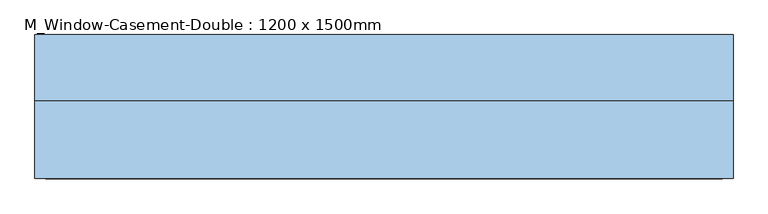
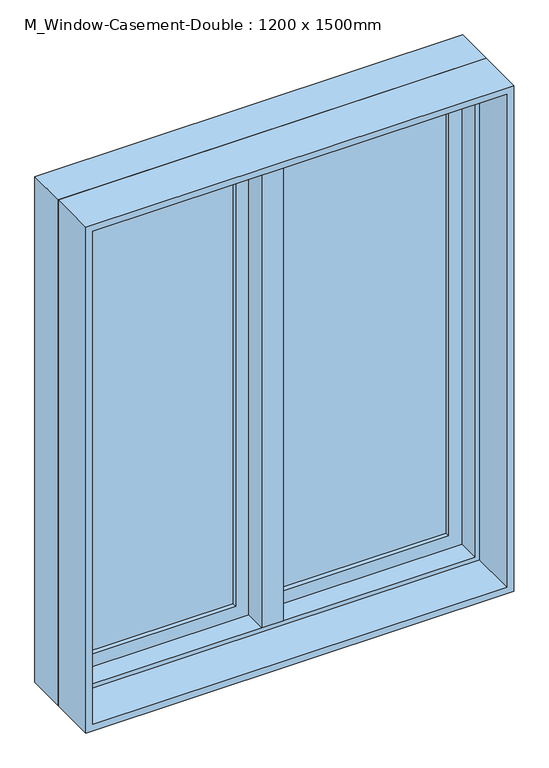
"""IFC4 building model written with IfcOpenShell, lengths in millimetres: window geometry, M_Window-Casement-Double : 1200 x 1500mm."""

from ifc_helpers import new_model, si_unit, frame, origin, place, context, project, spatial, polyline, outline, extrude, faceted_brep, source, transform, mapped, element, save


def m_window_casement_double_1200_x_1500mm_04159c99(model_context):
    return source(origin(), model_context, "Body", "SolidModel", [
        faceted_brep([(9.525, 133.35, 2387.3), (-9.525, 133.35, 2387.3), (-9.525, 82.55, 2387.3), (9.525, 82.55, 2387.3), (9.525, 133.35, 912.7), (9.525, 82.55, 912.7), (-9.525, 82.55, 912.7), (-9.525, 133.35, 912.7), (-9.525, 82.55, 931.75), (-9.525, 82.55, 2368.25), (-30.1625, 82.55, 931.75), (-30.1625, 82.55, 2368.25), (-30.1625, 19.05, 931.75), (-30.1625, 19.05, 2368.25), (30.1625, 19.05, 931.75), (30.1625, 19.05, 2368.25), (30.1625, 82.55, 931.75), (30.1625, 82.55, 2368.25), (9.525, 82.55, 931.75), (9.525, 82.55, 2368.25)], [[[0, 1, 2, 3]], [[4, 5, 6, 7]], [[1, 0, 4, 7]], [[2, 1, 7, 6, 8, 9]], [[9, 8, 10, 11]], [[11, 10, 12, 13]], [[13, 12, 14, 15]], [[15, 14, 16, 17]], [[17, 16, 18, 19]], [[0, 3, 19, 18, 5, 4]], [[18, 8, 6, 5]], [[9, 19, 3, 2]], [[8, 18, 16, 14, 12, 10]], [[19, 9, 11, 13, 15, 17]]]),
        extrude(outline(polyline([(-66.675, 114.3), (-66.675, 107.95), (-530.15, 107.95), (-530.15, 114.3), (-66.675, 114.3)])), frame((0.0, 0.0, 969.85), z_axis=(0.0, 0.0, 1.0), x_axis=(1.0, 0.0, 0.0)), (0.0, 0.0, 1.0), 1360.3),
        extrude(outline(polyline([(-530.15, 95.25), (-530.15, 101.6), (-66.675, 101.6), (-66.675, 95.25), (-530.15, 95.25)])), frame((0.0, 0.0, 969.85), z_axis=(0.0, 0.0, 1.0), x_axis=(1.0, 0.0, 0.0)), (0.0, 0.0, 1.0), 1360.3),
        extrude(outline(polyline([(530.15, 114.3), (530.15, 107.95), (66.675, 107.95), (66.675, 114.3), (530.15, 114.3)])), frame((0.0, 0.0, 969.85), z_axis=(0.0, 0.0, 1.0), x_axis=(1.0, 0.0, 0.0)), (0.0, 0.0, 1.0), 1360.3),
        extrude(outline(polyline([(66.675, 95.25), (66.675, 101.6), (530.15, 101.6), (530.15, 95.25), (66.675, 95.25)])), frame((0.0, 0.0, 969.85), z_axis=(0.0, 0.0, 1.0), x_axis=(1.0, 0.0, 0.0)), (0.0, 0.0, 1.0), 1360.3),
        extrude(outline(polyline([(2387.3, -587.3), (912.7, -587.3), (912.7, -9.525), (2387.3, -9.525), (2387.3, -587.3)]), holes=[polyline([(2330.15, -66.675), (969.85, -66.675), (969.85, -530.15), (2330.15, -530.15), (2330.15, -66.675)])]), frame((0.0, 82.55, 0.0), z_axis=(0.0, 1.0, 0.0), x_axis=(0.0, 0.0, 1.0)), (0.0, 0.0, 1.0), 44.45),
        extrude(outline(polyline([(912.7, 587.3), (2387.3, 587.3), (2387.3, 9.525), (912.7, 9.525), (912.7, 587.3)]), holes=[polyline([(969.85, 66.675), (2330.15, 66.675), (2330.15, 530.15), (969.85, 530.15), (969.85, 66.675)])]), frame((0.0, 82.55, 0.0), z_axis=(0.0, 1.0, 0.0), x_axis=(0.0, 0.0, 1.0)), (0.0, 0.0, 1.0), 44.45),
        extrude(outline(polyline([(2400.0, -600.0), (900.0, -600.0), (900.0, 600.0), (2400.0, 600.0), (2400.0, -600.0)]), holes=[polyline([(2380.95, 580.95), (919.05, 580.95), (919.05, -580.95), (2380.95, -580.95), (2380.95, 580.95)])]), frame((0.0, -114.3, 0.0), z_axis=(0.0, 1.0, 0.0), x_axis=(0.0, 0.0, 1.0)), (0.0, 0.0, 1.0), 133.35),
        faceted_brep([(568.25, 82.55, 2368.25), (568.25, 19.05, 2368.25), (-568.25, 19.05, 2368.25), (-568.25, 82.55, 2368.25), (587.3, 133.35, 2387.3), (587.3, 82.55, 2387.3), (-587.3, 82.55, 2387.3), (-587.3, 133.35, 2387.3), (600.0, 19.05, 2400.0), (600.0, 133.35, 2400.0), (-600.0, 133.35, 2400.0), (-600.0, 19.05, 2400.0), (-568.25, 19.05, 931.75), (-568.25, 82.55, 931.75), (-587.3, 82.55, 912.7), (-587.3, 133.35, 912.7), (-600.0, 133.35, 900.0), (-600.0, 19.05, 900.0), (568.25, 19.05, 931.75), (568.25, 82.55, 931.75), (587.3, 82.55, 912.7), (587.3, 133.35, 912.7), (600.0, 133.35, 900.0), (600.0, 19.05, 900.0)], [[[0, 1, 2, 3]], [[4, 5, 6, 7]], [[8, 9, 10, 11]], [[3, 2, 12, 13]], [[7, 6, 14, 15]], [[11, 10, 16, 17]], [[13, 12, 18, 19]], [[15, 14, 20, 21]], [[17, 16, 22, 23]], [[11, 17, 23, 8], [1, 18, 12, 2]], [[19, 18, 1, 0]], [[5, 20, 14, 6], [3, 13, 19, 0]], [[21, 20, 5, 4]], [[23, 22, 9, 8]], [[9, 22, 16, 10], [7, 15, 21, 4]]]),
    ])


if __name__ == "__main__":
    model = new_model("IFC4")
    model_context = context("Model", 3, world=origin())
    ifc_project = project(units=[si_unit("LENGTHUNIT", "METRE", prefix="MILLI")], contexts=[model_context])
    site = spatial("IfcSite", under=ifc_project)
    building = spatial("IfcBuilding", under=site)
    placement = place(None, origin())
    m_window_casement_double_1200_x_1500mm_shape = m_window_casement_double_1200_x_1500mm_04159c99(model_context)
    element("IfcWindow", 1, ObjectType="M_Window-Casement-Double : 1200 x 1500mm", at=placement, inside=building, context=model_context, shape_type="MappedRepresentation", body=[
        mapped(m_window_casement_double_1200_x_1500mm_shape, transform((0.0, 0.0, 0.0), x_axis=(1.0, 0.0, 0.0), y_axis=(0.0, 1.0, 0.0), z_axis=(0.0, 0.0, 1.0))),
    ])
    save(model, "model.ifc")

# Revit data of these elements
# Type "M_Window-Casement-Double : 1200 x 1500mm"
#   Type Mark = "25"
#   Fire Rating = "0.5h"
#   Assembly Code = "B2020100"
#   Analytic Construction = "Double glazing - domestic"
#   Frame Extension [instance default] = 0.020833 ft
#   Window Inset [instance default] = 0.0 ft
#   Wall Thickness [instance default] = 0.492126 ft
#   Interior Wall Closure [instance default] = 0.179626 ft
#   Half Width = 1.968504 ft
#   Visual Light Transmittance = 0.81
#   Thermal Resistance (R) = 0.319569 (m²·K)/W
#   Solar Heat Gain Coefficient = 0.76
#   Rough Width = 3.98622 ft
#   Rough Height = 4.970472 ft
#   Height = 4.92126 ft
#   Heat Transfer Coefficient (U) = 3.12929 W/(m²·K)
#   Exterior Wall Closure [instance default] = 0.104331 ft
#   Extension Jamb [instance default] = 0.179626 ft
#   Default Sill Height = 2.952756 ft
#   Width = 3.937008 ft
#   Define Thermal Properties by = 0
#   Muntin Visibility = yes
#   Interior Trim Visibility [instance default] = yes
#   Exterior Trim Visibility [instance default] = yes
#   Extension Jamb Visibility [instance default] = yes
#   Interior Trim Material = Wood - Stained
#   Muntin Pattern = M_Muntin Pattern_2x2 : M_Muntin Pattern_2x2
#   Interior Trim = M_Trim-Window-Interior-Flat : Picture Frame
#   Interior Frame Material = Wood - Stained
#   Glass Panel Material = Glass
#   Exterior Trim Material = Clad - White
#   Exterior Trim = M_Trim-Window-Exterior-Flat : with Sill
#   Exterior Frame Material = Clad - White
#   Wall Closure = (empty or 0)
# Element 1 (IfcWindow, "M_Window-Casement-Double : 1200 x 1500mm")
#   Wall Thickness = 0.75 ft
#   Extension Jamb = 0.4375 ft
#   Materials on its faces: "Wood - Stained", "Glass", "Clad - White"
# Materials
#   "Wood - Stained": class "Wood", colour RGB 224 178 126, transparency 0, Cost = 0
#   "Glass": class "Glass", colour RGB 0 128 192, transparency 0.9, Description = "Soda Lime Glass", Cost = 0
#   "Clad - White": class "Wood", colour RGB 242 242 238, transparency 0, Cost = 0
